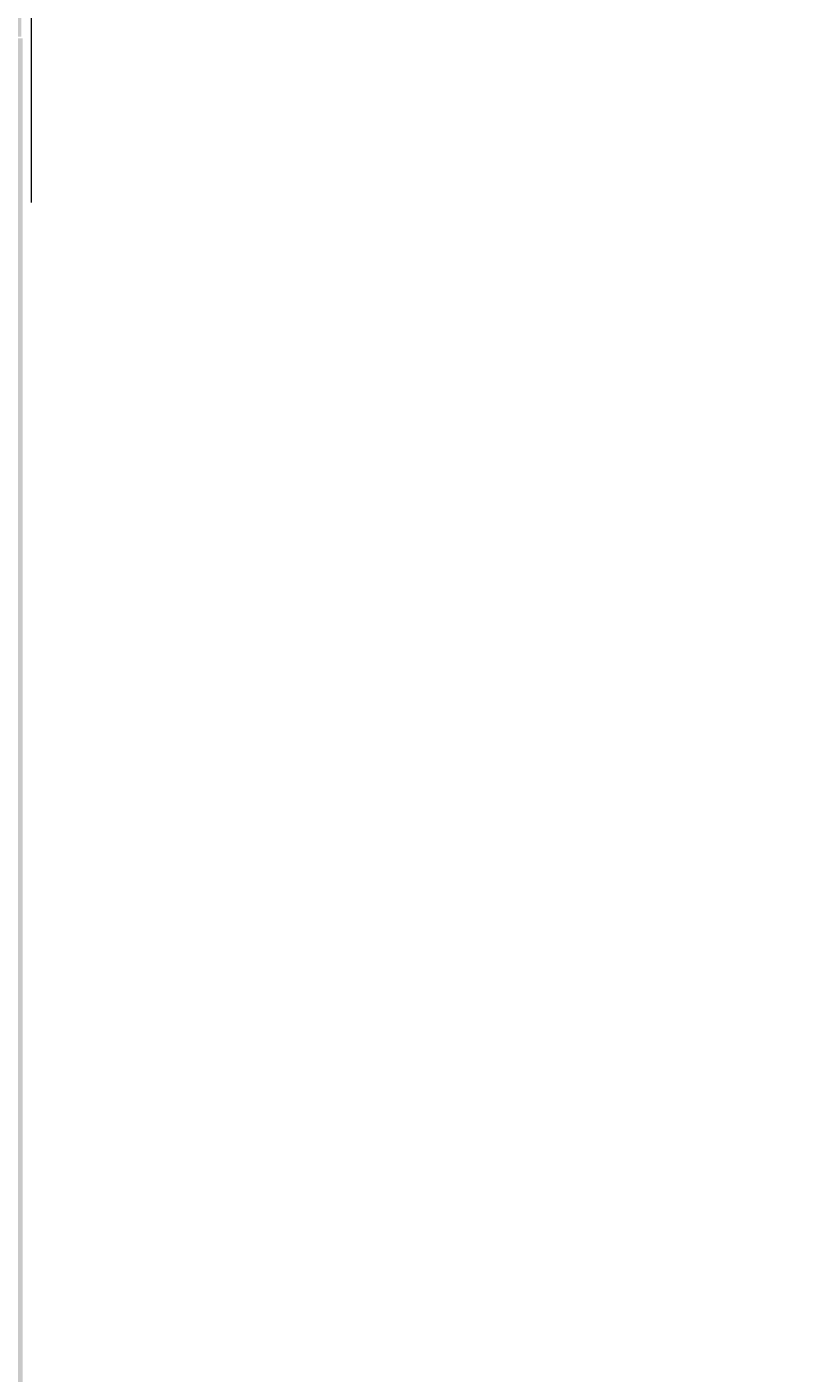
# Model space of a CAD drawing. Units: millimetres. Extents: x 27017497 to 27018854, y 7058029 to 7059154.
# Tile 71 of 91: x 27018341 to 27018360, y 7058174 to 7058207. Entities that reach past the tile are written whole.
import ezdxf

# ---------------------------------------------------------------- set-up
doc = ezdxf.new("R2010")
doc.units = ezdxf.units.MM
for name, color, linetype, lineweight in [('A-ANNO-DIMS', 2, 'Continuous', 18), ('A-FLOR-CASE', 8, 'Continuous', 20), ('A-FLOR-CASE-PATT', 44, 'Continuous', 13)]:
    doc.layers.add(name, color=color, linetype=linetype, lineweight=lineweight)
doc.styles.get("Standard").update_dxf_attribs({"font": 'arial.ttf'})
doc.dimstyles.get("Standard").update_dxf_attribs({"dimtxt": 0.18, "dimasz": 0.18, "dimexe": 0.18, "dimexo": 0.0625, "dimgap": 0.09, "dimtad": 0, "dimtih": 1, "dimtoh": 1, "dimdec": 4, "dimzin": 0, "dimdsep": 46, "dimtxsty": 'Standard', "dimcen": 0.09, "dimadec": 0, "dimazin": 0, "dimtfac": 1, "dimtdec": 4, "dimtofl": 0, "dimtmove": 0, "dimatfit": 3, "dimfxl": 1, "dimtolj": 1, "dimtzin": 0, "dimarcsym": 0})

# ---------------------------------------------------------------- blocks, each defined once
blk = doc.blocks.new('*D47')
at = {"layer": 'A-ANNO-DIMS', "color": 0, "lineweight": -2, "transparency": 16777216}
for p, q in [((27017561.166, 7058294.35), (27017561.166, 7058028.6)), ((27018790.606, 7058294.35), (27018790.606, 7058028.6)), ((27017561.346, 7058028.78), (27018175.431, 7058028.78)), ((27018790.426, 7058028.78), (27018176.341, 7058028.78))]:
    blk.add_line(p, q, dxfattribs=at)
at = {"layer": 'A-ANNO-DIMS', "color": 0, "transparency": 16777216}
for points in [[(27017561.346, 7058028.81), (27017561.346, 7058028.75), (27017561.166, 7058028.78)], [(27018790.426, 7058028.81), (27018790.426, 7058028.75), (27018790.606, 7058028.78)]]:
    blk.add_solid(points, dxfattribs=at)
at = {"layer": 'Defpoints', "color": 0, "transparency": 16777216}
for p in [(27017561.166, 7058294.412), (27018790.606, 7058294.412), (27018790.606, 7058028.78)]:
    blk.add_point(p, dxfattribs=at)
at = {"layer": 'A-ANNO-DIMS', "color": 0, "transparency": 16777216, "insert": (27018175.886, 7058028.78), "char_height": 0.18, "attachment_point": 5}
blk.add_mtext('\\A1;1229.4', dxfattribs=at)
blk = doc.blocks.new('*D48')
at = {"layer": 'A-ANNO-DIMS', "color": 0, "lineweight": -2, "transparency": 16777216}
for p, q in [((27018463.498, 7058622.912), (27017497.536, 7058622.912)), ((27017497.716, 7058622.732), (27017497.716, 7058357.753)), ((27017497.716, 7058092.41), (27017497.716, 7058357.389)), ((27018555.129, 7058092.23), (27017497.536, 7058092.23))]:
    blk.add_line(p, q, dxfattribs=at)
at = {"layer": 'A-ANNO-DIMS', "color": 0, "transparency": 16777216}
for points in [[(27017497.686, 7058622.732), (27017497.746, 7058622.732), (27017497.716, 7058622.912)], [(27017497.686, 7058092.41), (27017497.746, 7058092.41), (27017497.716, 7058092.23)]]:
    blk.add_solid(points, dxfattribs=at)
at = {"layer": 'Defpoints', "color": 0, "transparency": 16777216}
for p in [(27018463.561, 7058622.912), (27017497.716, 7058092.23), (27018555.192, 7058092.23)]:
    blk.add_point(p, dxfattribs=at)
at = {"layer": 'A-ANNO-DIMS', "color": 0, "transparency": 16777216, "insert": (27017497.716, 7058357.571), "char_height": 0.18, "attachment_point": 5}
blk.add_mtext('\\A1;530.7', dxfattribs=at)

msp = doc.modelspace()

# ---------------------------------------------------------------- hatches: boundary and pattern name
at = {"layer": 'A-FLOR-CASE-PATT'}
h = msp.add_hatch(color=256, dxfattribs=at)
h.dxf.hatch_style = 1
edge = h.paths.add_edge_path()
edge.add_line((27018341.343, 7058207.055), (27018330.837, 7058207.055))
edge.add_line((27018330.837, 7058207.055), (27018330.837, 7058203.02))
edge.add_line((27018330.837, 7058203.02), (27018338.424, 7058203.02))
edge.add_ellipse((27018338.23, 7058202.551), major_axis=(0.528, 0), ratio=0.888892, start_angle=0, end_angle=90, ccw=False)
edge.add_line((27018338.758, 7058202.551), (27018338.758, 7058202.238))
edge.add_line((27018338.758, 7058202.238), (27018330.837, 7058201.488))
edge.add_line((27018330.837, 7058201.488), (27018330.837, 7058199.747))
edge.add_line((27018330.837, 7058199.747), (27018338.424, 7058199.747))
edge.add_ellipse((27018338.23, 7058199.277), major_axis=(0.528, 0), ratio=0.888892, start_angle=0, end_angle=90, ccw=False)
edge.add_line((27018338.758, 7058199.277), (27018338.758, 7058198.964))
edge.add_line((27018338.758, 7058198.964), (27018330.837, 7058198.215))
edge.add_line((27018330.837, 7058198.215), (27018330.837, 7058193.415))
edge.add_line((27018330.837, 7058193.415), (27018338.284, 7058190.704))
edge.add_ellipse((27018337.942, 7058190.329), major_axis=(0.496, -0.181), ratio=0.888892, start_angle=0, end_angle=90, ccw=False)
edge.add_line((27018338.439, 7058190.148), (27018338.331, 7058189.854))
edge.add_line((27018338.331, 7058189.854), (27018330.837, 7058191.806))
edge.add_line((27018330.837, 7058191.806), (27018330.837, 7058188.22))
edge.add_line((27018330.837, 7058188.22), (27018338.424, 7058188.22))
edge.add_ellipse((27018338.23, 7058187.75), major_axis=(0.528, 0), ratio=0.888892, start_angle=0, end_angle=90, ccw=False)
edge.add_line((27018338.758, 7058187.75), (27018338.758, 7058187.437))
edge.add_line((27018338.758, 7058187.437), (27018330.837, 7058186.688))
edge.add_line((27018330.837, 7058186.688), (27018330.837, 7058181.982))
edge.add_line((27018330.837, 7058181.982), (27018338.424, 7058181.982))
edge.add_ellipse((27018338.23, 7058181.513), major_axis=(0.528, 0), ratio=0.888892, start_angle=0, end_angle=90, ccw=False)
edge.add_line((27018338.758, 7058181.513), (27018338.758, 7058181.199))
edge.add_line((27018338.758, 7058181.199), (27018330.837, 7058180.45))
edge.add_line((27018330.837, 7058180.45), (27018330.837, 7058178.709))
edge.add_line((27018330.837, 7058178.709), (27018338.424, 7058178.709))
edge.add_ellipse((27018338.23, 7058178.239), major_axis=(0.528, 0), ratio=0.888892, start_angle=0, end_angle=90, ccw=False)
edge.add_line((27018338.758, 7058178.239), (27018338.758, 7058177.926))
edge.add_line((27018338.758, 7058177.926), (27018330.837, 7058177.177))
edge.add_line((27018330.837, 7058177.177), (27018330.837, 7058173.878))
edge.add_line((27018330.837, 7058173.878), (27018338.284, 7058171.167))
edge.add_ellipse((27018337.942, 7058170.792), major_axis=(0.496, -0.181), ratio=0.888892, start_angle=0, end_angle=90, ccw=False)
edge.add_line((27018338.439, 7058170.611), (27018338.331, 7058170.317))
edge.add_line((27018338.331, 7058170.317), (27018330.837, 7058172.269))
edge.add_line((27018330.837, 7058172.269), (27018330.837, 7058168.293))
edge.add_line((27018330.837, 7058168.293), (27018338.424, 7058168.293))
edge.add_ellipse((27018338.23, 7058167.824), major_axis=(0.528, 0), ratio=0.888892, start_angle=0, end_angle=90, ccw=False)
edge.add_line((27018338.758, 7058167.824), (27018338.758, 7058167.511))
edge.add_line((27018338.758, 7058167.511), (27018330.837, 7058166.762))
edge.add_line((27018330.837, 7058166.762), (27018330.837, 7058160.389))
edge.add_line((27018330.837, 7058160.389), (27018338.424, 7058160.389))
edge.add_ellipse((27018338.23, 7058159.92), major_axis=(0.528, 0), ratio=0.888892, start_angle=0, end_angle=90, ccw=False)
edge.add_line((27018338.758, 7058159.92), (27018338.758, 7058159.607))
edge.add_line((27018338.758, 7058159.607), (27018330.837, 7058158.858))
edge.add_line((27018330.837, 7058158.858), (27018330.837, 7058157.116))
edge.add_line((27018330.837, 7058157.116), (27018338.424, 7058157.116))
edge.add_ellipse((27018338.23, 7058156.647), major_axis=(0.528, 0), ratio=0.888892, start_angle=0, end_angle=90, ccw=False)
edge.add_line((27018338.758, 7058156.647), (27018338.758, 7058156.334))
edge.add_line((27018338.758, 7058156.334), (27018330.837, 7058155.585))
edge.add_line((27018330.837, 7058155.585), (27018330.837, 7058150.784))
edge.add_line((27018330.837, 7058150.784), (27018338.284, 7058148.073))
edge.add_ellipse((27018337.942, 7058147.698), major_axis=(0.496, -0.181), ratio=0.888892, start_angle=0, end_angle=90, ccw=False)
edge.add_line((27018338.439, 7058147.517), (27018338.331, 7058147.223))
edge.add_line((27018338.331, 7058147.223), (27018330.837, 7058149.175))
edge.add_line((27018330.837, 7058149.175), (27018330.837, 7058145.589))
edge.add_line((27018330.837, 7058145.589), (27018338.424, 7058145.589))
edge.add_ellipse((27018338.23, 7058145.119), major_axis=(0.528, 0), ratio=0.888892, start_angle=0, end_angle=90, ccw=False)
edge.add_line((27018338.758, 7058145.119), (27018338.758, 7058144.806))
edge.add_line((27018338.758, 7058144.806), (27018330.837, 7058144.057))
edge.add_line((27018330.837, 7058144.057), (27018330.837, 7058141.912))
edge.add_line((27018330.837, 7058141.912), (27018341.343, 7058141.912))
edge.add_line((27018341.343, 7058141.912), (27018341.343, 7058207.055))
edge = h.paths.add_edge_path()
edge.add_line((27018330.112, 7058207.055), (27018319.606, 7058207.055))
edge.add_line((27018319.606, 7058207.055), (27018319.606, 7058141.912))
edge.add_line((27018319.606, 7058141.912), (27018330.112, 7058141.912))
edge.add_line((27018330.112, 7058141.912), (27018330.112, 7058144.024))
edge.add_line((27018330.112, 7058144.024), (27018322.543, 7058144.024))
edge.add_ellipse((27018322.736, 7058144.493), major_axis=(0.528, 0), ratio=0.888892, start_angle=180, end_angle=270, ccw=False)
edge.add_line((27018322.208, 7058144.493), (27018322.208, 7058145.291))
edge.add_ellipse((27018322.736, 7058145.119), major_axis=(0.528, 0), ratio=0.888892, start_angle=90, end_angle=180, ccw=False)
edge.add_line((27018322.736, 7058145.589), (27018330.112, 7058145.589))
edge.add_line((27018330.112, 7058145.589), (27018330.112, 7058149.382))
edge.add_line((27018330.112, 7058149.382), (27018322.826, 7058152.034))
edge.add_ellipse((27018323.168, 7058152.409), major_axis=(0.496, -0.181), ratio=0.888892, start_angle=180, end_angle=270, ccw=False)
edge.add_line((27018322.672, 7058152.59), (27018322.945, 7058153.34))
edge.add_ellipse((27018323.382, 7058152.997), major_axis=(0.496, -0.181), ratio=0.888892, start_angle=90, end_angle=180, ccw=False)
edge.add_line((27018323.543, 7058153.439), (27018330.112, 7058151.048))
edge.add_line((27018330.112, 7058151.048), (27018330.112, 7058155.551))
edge.add_line((27018330.112, 7058155.551), (27018322.543, 7058155.551))
edge.add_ellipse((27018322.736, 7058156.021), major_axis=(0.528, 0), ratio=0.888892, start_angle=180, end_angle=270, ccw=False)
edge.add_line((27018322.208, 7058156.021), (27018322.208, 7058156.819))
edge.add_ellipse((27018322.736, 7058156.647), major_axis=(0.528, 0), ratio=0.888892, start_angle=90, end_angle=180, ccw=False)
edge.add_line((27018322.736, 7058157.116), (27018330.112, 7058157.116))
edge.add_line((27018330.112, 7058157.116), (27018330.112, 7058158.824))
edge.add_line((27018330.112, 7058158.824), (27018322.543, 7058158.824))
edge.add_ellipse((27018322.736, 7058159.294), major_axis=(0.528, 0), ratio=0.888892, start_angle=180, end_angle=270, ccw=False)
edge.add_line((27018322.208, 7058159.294), (27018322.208, 7058160.092))
edge.add_ellipse((27018322.736, 7058159.92), major_axis=(0.528, 0), ratio=0.888892, start_angle=90, end_angle=180, ccw=False)
edge.add_line((27018322.736, 7058160.389), (27018330.112, 7058160.389))
edge.add_line((27018330.112, 7058160.389), (27018330.112, 7058166.728))
edge.add_line((27018330.112, 7058166.728), (27018322.543, 7058166.728))
edge.add_ellipse((27018322.736, 7058167.198), major_axis=(0.528, 0), ratio=0.888892, start_angle=180, end_angle=270, ccw=False)
edge.add_line((27018322.208, 7058167.198), (27018322.208, 7058167.996))
edge.add_ellipse((27018322.736, 7058167.824), major_axis=(0.528, 0), ratio=0.888892, start_angle=90, end_angle=180, ccw=False)
edge.add_line((27018322.736, 7058168.293), (27018330.112, 7058168.293))
edge.add_line((27018330.112, 7058168.293), (27018330.112, 7058172.476))
edge.add_line((27018330.112, 7058172.476), (27018322.826, 7058175.128))
edge.add_ellipse((27018323.168, 7058175.503), major_axis=(0.496, -0.181), ratio=0.888892, start_angle=180, end_angle=270, ccw=False)
edge.add_line((27018322.672, 7058175.684), (27018322.945, 7058176.433))
edge.add_ellipse((27018323.382, 7058176.091), major_axis=(0.496, -0.181), ratio=0.888892, start_angle=90, end_angle=180, ccw=False)
edge.add_line((27018323.543, 7058176.533), (27018330.112, 7058174.142))
edge.add_line((27018330.112, 7058174.142), (27018330.112, 7058177.144))
edge.add_line((27018330.112, 7058177.144), (27018322.543, 7058177.144))
edge.add_ellipse((27018322.736, 7058177.613), major_axis=(0.528, 0), ratio=0.888892, start_angle=180, end_angle=270, ccw=False)
edge.add_line((27018322.208, 7058177.613), (27018322.208, 7058178.411))
edge.add_ellipse((27018322.736, 7058178.239), major_axis=(0.528, 0), ratio=0.888892, start_angle=90, end_angle=180, ccw=False)
edge.add_line((27018322.736, 7058178.709), (27018330.112, 7058178.709))
edge.add_line((27018330.112, 7058178.709), (27018330.112, 7058180.417))
edge.add_line((27018330.112, 7058180.417), (27018322.543, 7058180.417))
edge.add_ellipse((27018322.736, 7058180.886), major_axis=(0.528, 0), ratio=0.888892, start_angle=180, end_angle=270, ccw=False)
edge.add_line((27018322.208, 7058180.886), (27018322.208, 7058181.684))
edge.add_ellipse((27018322.736, 7058181.513), major_axis=(0.528, 0), ratio=0.888892, start_angle=90, end_angle=180, ccw=False)
edge.add_line((27018322.736, 7058181.982), (27018330.112, 7058181.982))
edge.add_line((27018330.112, 7058181.982), (27018330.112, 7058186.655))
edge.add_line((27018330.112, 7058186.655), (27018322.543, 7058186.655))
edge.add_ellipse((27018322.736, 7058187.124), major_axis=(0.528, 0), ratio=0.888892, start_angle=180, end_angle=270, ccw=False)
edge.add_line((27018322.208, 7058187.124), (27018322.208, 7058187.922))
edge.add_ellipse((27018322.736, 7058187.75), major_axis=(0.528, 0), ratio=0.888892, start_angle=90, end_angle=180, ccw=False)
edge.add_line((27018322.736, 7058188.22), (27018330.112, 7058188.22))
edge.add_line((27018330.112, 7058188.22), (27018330.112, 7058192.013))
edge.add_line((27018330.112, 7058192.013), (27018322.826, 7058194.665))
edge.add_ellipse((27018323.168, 7058195.04), major_axis=(0.496, -0.181), ratio=0.888892, start_angle=180, end_angle=270, ccw=False)
edge.add_line((27018322.672, 7058195.22), (27018322.945, 7058195.97))
edge.add_ellipse((27018323.382, 7058195.628), major_axis=(0.496, -0.181), ratio=0.888892, start_angle=90, end_angle=180, ccw=False)
edge.add_line((27018323.543, 7058196.069), (27018330.112, 7058193.678))
edge.add_line((27018330.112, 7058193.678), (27018330.112, 7058198.182))
edge.add_line((27018330.112, 7058198.182), (27018322.543, 7058198.182))
edge.add_ellipse((27018322.736, 7058198.651), major_axis=(0.528, 0), ratio=0.888892, start_angle=180, end_angle=270, ccw=False)
edge.add_line((27018322.208, 7058198.651), (27018322.208, 7058199.449))
edge.add_ellipse((27018322.736, 7058199.277), major_axis=(0.528, 0), ratio=0.888892, start_angle=90, end_angle=180, ccw=False)
edge.add_line((27018322.736, 7058199.747), (27018330.112, 7058199.747))
edge.add_line((27018330.112, 7058199.747), (27018330.112, 7058201.455))
edge.add_line((27018330.112, 7058201.455), (27018322.543, 7058201.455))
edge.add_ellipse((27018322.736, 7058201.924), major_axis=(0.528, 0), ratio=0.888892, start_angle=180, end_angle=270, ccw=False)
edge.add_line((27018322.208, 7058201.924), (27018322.208, 7058202.722))
edge.add_ellipse((27018322.736, 7058202.551), major_axis=(0.528, 0), ratio=0.888892, start_angle=90, end_angle=180, ccw=False)
edge.add_line((27018322.736, 7058203.02), (27018330.112, 7058203.02))
edge.add_line((27018330.112, 7058203.02), (27018330.112, 7058207.055))
h.paths.add_polyline_path([(27018341.31, 7058294.412), (27018319.606, 7058294.412), (27018319.606, 7058207.1), (27018341.31, 7058207.1)])
h.paths.add_polyline_path([(27018354.358, 7058255.592), (27018354.358, 7058256.057, -0.414214), (27018354.869, 7058256.569), (27018346.477, 7058256.569, -0.414214), (27018345.197, 7058257.848), (27018345.197, 7058259.128, -0.414214), (27018346.477, 7058260.407), (27018343.868, 7058260.407, 0.290979), (27018341.551, 7058258.934), (27018341.551, 7058242.534, 0.290979), (27018343.868, 7058241.06), (27018346.477, 7058241.06, -0.414214), (27018345.197, 7058242.34), (27018345.197, 7058243.619, -0.414214), (27018346.477, 7058244.899), (27018353.078, 7058244.899, 0.414214), (27018354.358, 7058246.178)])
h.paths.add_polyline_path([(27018356.917, 7058260.407), (27018346.477, 7058260.407, 0.414214), (27018345.197, 7058259.128), (27018345.197, 7058257.848, 0.414214), (27018346.477, 7058256.569), (27018355.637, 7058256.569), (27018355.637, 7058244.899), (27018346.477, 7058244.899, 0.414214), (27018345.197, 7058243.619), (27018345.197, 7058242.34, 0.414214), (27018346.477, 7058241.06), (27018356.917, 7058241.06, 0.414214), (27018359.476, 7058243.619), (27018359.476, 7058257.848, 0.414214)])
h.paths.add_polyline_path([(27018355.637, 7058252.362), (27018355.637, 7058256.057, 0.490314), (27018354.997, 7058256.553, 0.490314), (27018354.358, 7058256.057), (27018354.358, 7058255.592), (27018354.358, 7058245.411, 0.490314), (27018354.997, 7058244.915, 0.490314), (27018355.637, 7058245.411)], flags=17)

# ---------------------------------------------------------------- linework, layer by layer
at = {"layer": 'A-FLOR-CASE'}
msp.add_line((27018341.551, 7058290.392), (27018341.551, 7058203.035), dxfattribs=at)

# ---------------------------------------------------------------- dimensions: what is measured, and where the dimension line sits
at = {"layer": 'A-ANNO-DIMS'}
dim = msp.add_linear_dim(base=(27017497.716, 7058092.23), p1=(27018463.561, 7058622.912), p2=(27018555.192, 7058092.23), angle=90, dimstyle='Standard', override={"dimdec": 1, "dimlfac": 1, "dimrnd": 0, "dimzin": 0, "dimdsep": 46, "dimlunit": 2}, dxfattribs=at)
dim.commit()
dim.dimension.update_dxf_attribs({"geometry": '*D48', "text_midpoint": (27017497.716, 7058357.571)})
dim = msp.add_linear_dim(base=(27018790.606, 7058028.78), p1=(27017561.166, 7058294.412), p2=(27018790.606, 7058294.412), dimstyle='Standard', override={"dimdec": 1, "dimlfac": 1, "dimrnd": 0, "dimzin": 0, "dimdsep": 46, "dimlunit": 2}, dxfattribs=at)
dim.commit()
dim.dimension.update_dxf_attribs({"geometry": '*D47', "text_midpoint": (27018175.886, 7058028.78)})

doc.saveas('drawing.dxf')
